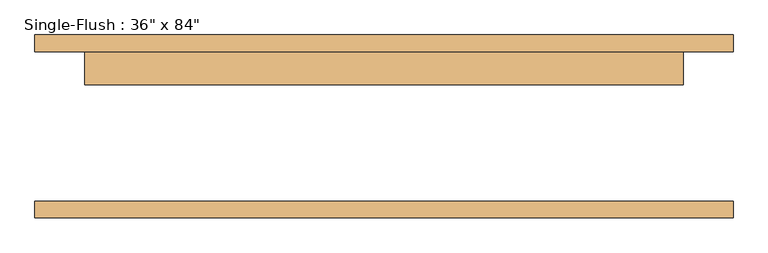
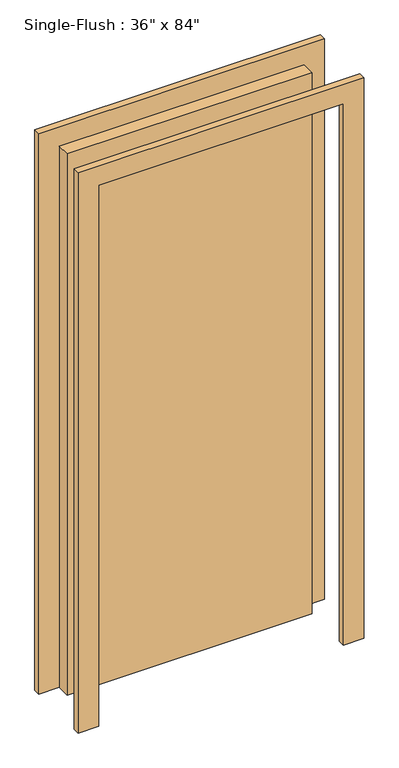
"""IFC4 building model written with IfcOpenShell, lengths in millimetres: door geometry."""

from ifc_helpers import new_model, si_unit, frame, origin, origin_with_axes, place, context, project, spatial, polyline, outline, extrude, source, transform, mapped, element, save


def door_0ca8825f(model_context):
    return source(origin(), model_context, "Body", "SweptSolid", [
        extrude(outline(polyline([(2209.8, -533.4), (0.0, -533.4), (0.0, -457.2), (2133.6, -457.2), (2133.6, 457.2), (0.0, 457.2), (0.0, 533.4), (2209.8, 533.4), (2209.8, -533.4)])), frame((0.0, 114.3, 0.0), z_axis=(0.0, 1.0, 0.0), x_axis=(0.0, 0.0, 1.0)), (0.0, 0.0, 1.0), 25.4),
        extrude(outline(polyline([(2209.8, 533.4), (2209.8, -533.4), (0.0, -533.4), (0.0, -457.2), (2133.6, -457.2), (2133.6, 457.2), (0.0, 457.2), (0.0, 533.4), (2209.8, 533.4)])), frame((0.0, -139.7, 0.0), z_axis=(0.0, 1.0, 0.0), x_axis=(0.0, 0.0, 1.0)), (0.0, 0.0, 1.0), 25.4),
        extrude(outline(polyline([(457.2, 63.5), (-457.2, 63.5), (-457.2, 114.3), (457.2, 114.3), (457.2, 63.5)])), origin_with_axes(), (0.0, 0.0, 1.0), 2133.6),
    ])


if __name__ == "__main__":
    model = new_model("IFC4")
    model_context = context("Model", 3, world=origin())
    ifc_project = project(units=[si_unit("LENGTHUNIT", "METRE", prefix="MILLI")], contexts=[model_context])
    site = spatial("IfcSite", under=ifc_project)
    building = spatial("IfcBuilding", under=site)
    placement = place(None, origin())
    door_shape = door_0ca8825f(model_context)
    element("IfcDoor", 1, ObjectType="Single-Flush : 36\" x 84\"", at=placement, inside=building, context=model_context, shape_type="MappedRepresentation", body=[
        mapped(door_shape, transform((0.0, 0.0, 0.0), x_axis=(1.0, 0.0, 0.0), y_axis=(0.0, 1.0, 0.0), z_axis=(0.0, 0.0, 1.0))),
    ])
    save(model, "model.ifc")

# Revit data of these elements
# Type "Single-Flush : 36\" x 84\""
#   Type Mark = "1"
#   Construction Type Id = "MDOOR"
#   Assembly Code = "C1020"
#   Analytic Construction = "Metal"
#   Thickness = 0' - 2"
#   Heat Transfer Coefficient (U) = 0.651978 BTU/(h·ft²·°F)
#   Height = 7' - 0"
#   Trim Projection Ext = 0' - 1"
#   Trim Projection Int = 0' - 1"
#   Trim Width = 0' - 3"
#   Width = 3' - 0"
#   Define Thermal Properties by = 1
#   Define Thermal Properties by = 1
#   Door Material = door
#   Frame Material = door
#   Visual Light Transmittance = 0
#   Solar Heat Gain Coefficient = 0
#   Function = (empty or 0)
#   Wall Closure = (empty or 0)
# Element 1 (IfcDoor, "Single-Flush : 36\" x 84\"")
#   Materials on its faces: "door"
# Materials
#   "door": class "Generic", colour RGB 120 120 120, transparency 0, Cost = 0
